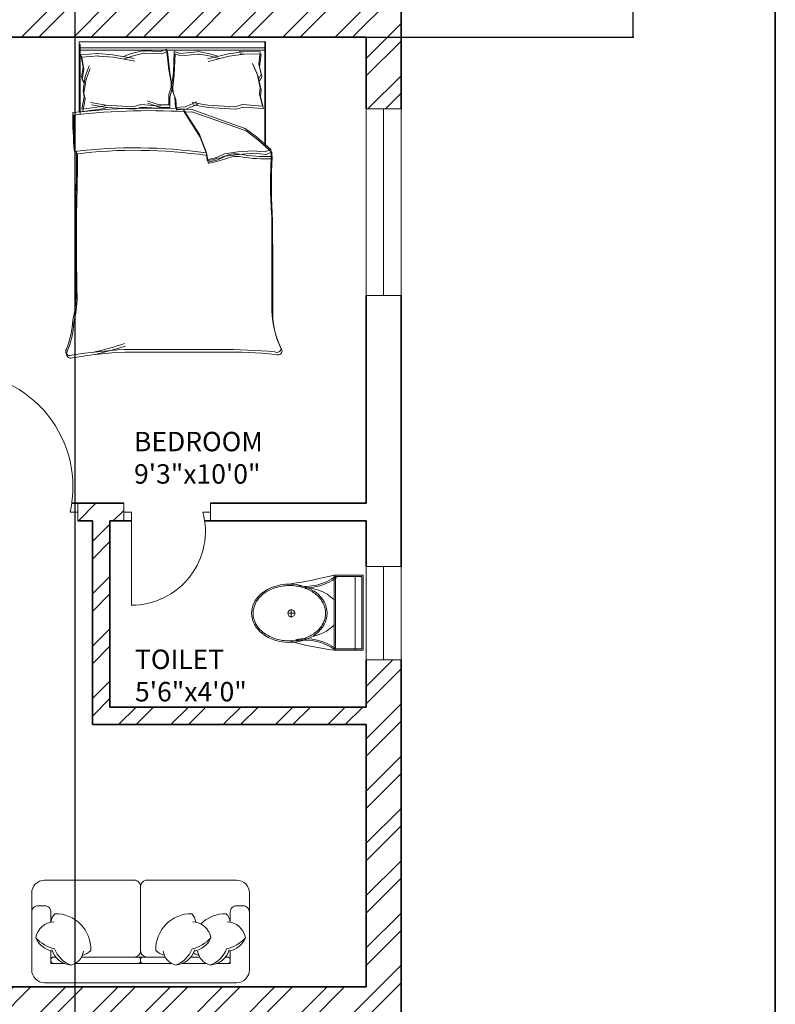
# Model space of a CAD drawing. Units: inches. Extents: x 2552 to 3217, y 1417 to 2737.
# Tile 13 of 25: x 3022 to 3217, y 1885 to 2138. Entities that reach past the tile are written whole.
import ezdxf

# ---------------------------------------------------------------- set-up
doc = ezdxf.new("R2010")
doc.units = ezdxf.units.IN
for name, color, linetype, lineweight in [('A-ANNO-DIMS', 2, 'Continuous', 18), ('A-ANNO-TTLB', 7, 'Continuous', 35), ('A-AREA-IDEN', 7, 'Continuous', 18), ('A-DOOR', 21, 'Continuous', 18), ('A-FLOR-FIXT', 8, 'Continuous', 18), ('A-FURN', 8, 'Continuous', 13), ('A-GLAZ', 161, 'Continuous', 18), ('A-WALL', 7, 'Continuous', 35), ('A-WALL-PATT', 217, 'Continuous', 13)]:
    doc.layers.add(name, color=color, linetype=linetype, lineweight=lineweight)
doc.styles.get("Standard").update_dxf_attribs({"font": 'arial.ttf'})
doc.dimstyles.get("Standard").update_dxf_attribs({"dimtxt": 0.18, "dimasz": 0.18, "dimexe": 0.18, "dimexo": 0.0625, "dimgap": 0.09, "dimtad": 0, "dimtih": 1, "dimtoh": 1, "dimdec": 4, "dimzin": 0, "dimdsep": 46, "dimtxsty": 'Standard', "dimcen": 0.09, "dimadec": 0, "dimazin": 0, "dimtfac": 1, "dimtdec": 4, "dimtofl": 0, "dimtmove": 0, "dimatfit": 3, "dimfxl": 1, "dimtolj": 1, "dimtzin": 0, "dimarcsym": 0})

# ---------------------------------------------------------------- blocks, each defined once
blk = doc.blocks.new('A$C31115884')
for p, q in [((283.1, 497.7), (223.4, 497.7)), ((257.5, 466.4), (257.5, 523.2)), ((0, 200), (0, 0)), ((520, 200), (0, 200)), ((10, 190), (10, 10)), ((510, 190), (10, 190)), ((510, 10), (510, 190)), ((520, 0), (520, 200)), ((510, 54.5), (0, 54.5)), ((10, 10), (510, 10)), ((0, 0), (520, 0))]:
    blk.add_line(p, q)
blk.add_circle((255.6, 496.4), 23.6)
for centre, radius, start, end in [((2777.7, -204.6), 2807, 165.4549, 171.71327), ((3237, 905), 2807, 188.28673, 194.5451), ((-294.5, 403.3), 364.7, 324.20913, 9.34987), ((-294.5, 403.3), 374.7, 324.20913, 9.34987), ((139.5, 406.2), 293.5, 315.84364, 2.65635), ((805.8, 403.3), 374.7, 179.20365, 215.79087), ((805.8, 403.3), 364.7, 170.65013, 215.79087), ((383.6, 406.2), 293.5, 190.27735, 224.15636)]:
    blk.add_arc(centre, radius, start, end)
blk.add_ellipse((256.2, 509.9), major_axis=(0, -260.7), ratio=0.772727)
blk.add_open_spline([(256.2, 259.2), (263.1, 259.2), (270, 259.7), (287.8, 262.3), (298.7, 265.1), (319.9, 273.1), (330.2, 278.4), (350.1, 291.1), (359.7, 298.7), (377.7, 315.9), (386.2, 325.5), (401.7, 346.6), (408.8, 358.1), (421.3, 382.5), (426.8, 395.5), (435.9, 422.4), (439.5, 436.4), (444.8, 465.1), (446.5, 479.7), (447.9, 509.2), (447.6, 524), (445, 553.3), (442.7, 567.8), (436.3, 596), (432.1, 609.7), (421.9, 636), (416, 648.6), (402.5, 672.1), (395, 683), (378.6, 703), (369.8, 712.1), (351.1, 728), (341.3, 734.8), (320.9, 746.2), (310.4, 750.7), (288.9, 757.3), (278, 759.4), (256, 761), (245, 760.6), (223.1, 757.2), (212.3, 754.3), (191.1, 746.1), (180.8, 740.7), (160.9, 727.8), (151.4, 720.1), (133.5, 702.7), (125.1, 693), (109.6, 671.7), (102.6, 660.2), (90.2, 635.7), (84.9, 622.7), (76, 595.6), (72.4, 581.6), (67.2, 552.9), (65.6, 538.2), (64.4, 508.8), (64.8, 494), (67.5, 464.7), (69.9, 450.2), (76.6, 422), (80.8, 408.3), (91.1, 382.2), (97.2, 369.7), (110.8, 346.3), (118.4, 335.4), (134.8, 315.6), (143.7, 306.7), (162.4, 290.9), (172.3, 284.2), (192.8, 273), (203.3, 268.6), (224.8, 262.2), (235.8, 260.2), (249.9, 259.3), (253, 259.2), (256.2, 259.2)], degree=3, knots=[0, 0, 0, 0, 0.110105, 0.110105, 0.285049, 0.285049, 0.459994, 0.459994, 0.634938, 0.634938, 0.809882, 0.809882, 0.984827, 0.984827, 1.159771, 1.159771, 1.334715, 1.334715, 1.50966, 1.50966, 1.684604, 1.684604, 1.859549, 1.859549, 2.034493, 2.034493, 2.209437, 2.209437, 2.384382, 2.384382, 2.559326, 2.559326, 2.73427, 2.73427, 2.909215, 2.909215, 3.084159, 3.084159, 3.259103, 3.259103, 3.434048, 3.434048, 3.608992, 3.608992, 3.783936, 3.783936, 3.958881, 3.958881, 4.133825, 4.133825, 4.30877, 4.30877, 4.483714, 4.483714, 4.658658, 4.658658, 4.833603, 4.833603, 5.008547, 5.008547, 5.183491, 5.183491, 5.358436, 5.358436, 5.53338, 5.53338, 5.708324, 5.708324, 5.883269, 5.883269, 6.058213, 6.058213, 6.233158, 6.233158, 6.283185, 6.283185, 6.283185, 6.283185])
blk = doc.blocks.new('BED-DOUBLE')
for p, q in [((3.47, 63.33), (3.47, 81.44)), ((3.47, 81.44), (51.49, 81.44)), ((3.48, 63.33), (3.48, 81.44)), ((51.27, 81.44), (51.27, 54.83)), ((51.27, 81.44), (51.27, 54.83)), ((51.49, 81.44), (51.49, 80.8)), ((3.47, 79.91), (51.27, 79.91)), ((3.48, 79.91), (51.27, 79.91)), ((3.7, 62.69), (3.7, 80.8)), ((3.7, 62.69), (3.7, 80.8)), ((3.7, 79.27), (51.49, 79.27)), ((3.7, 79.27), (51.49, 79.27)), ((16.88, 78.42), (19.77, 79.14)), ((16.88, 78.42), (19.77, 79.14)), ((19.77, 79.14), (20.09, 79.14)), ((19.77, 79.14), (20.09, 79.14)), ((20.09, 79.14), (24.54, 78.99)), ((20.09, 79.14), (24.54, 78.99)), ((24.54, 78.99), (25.98, 79.57)), ((24.54, 78.99), (25.98, 79.57)), ((24.77, 78.36), (26.21, 78.93)), ((24.77, 78.36), (26.21, 78.93)), ((25.98, 79.57), (26.56, 74.22)), ((25.98, 79.57), (26.56, 74.22)), ((26.21, 78.93), (26.79, 73.58)), ((26.21, 78.93), (26.79, 73.58)), ((27.98, 78.95), (27.73, 73.58)), ((27.98, 78.95), (27.73, 73.58)), ((29.46, 78.46), (27.98, 78.95)), ((29.46, 78.46), (27.98, 78.95)), ((33.88, 78.89), (29.46, 78.46)), ((33.88, 78.89), (29.46, 78.46)), ((34.2, 78.91), (33.88, 78.89)), ((34.2, 78.91), (33.88, 78.89)), ((37.14, 78.36), (34.2, 78.91)), ((37.14, 78.36), (34.2, 78.91)), ((45.71, 78.9), (41.91, 78.37)), ((45.71, 78.9), (41.91, 78.37)), ((50.11, 78.89), (44.71, 78.98)), ((44.71, 78.98), (45.71, 78.9)), ((50.11, 78.89), (44.71, 78.98)), ((44.71, 78.98), (45.71, 78.9)), ((50.11, 78.89), (49.73, 75.68)), ((50.11, 78.89), (49.73, 75.68)), ((51.49, 80.8), (51.49, 54.19)), ((51.49, 80.8), (51.49, 54.19)), ((3.89, 78.13), (4.47, 74.95)), ((3.89, 78.13), (4.47, 74.95)), ((3.9, 78.11), (8.18, 78.43)), ((3.9, 78.11), (8.18, 78.43)), ((4.12, 77.49), (4.7, 74.31)), ((4.12, 77.49), (4.7, 74.31)), ((4.13, 77.47), (8.41, 77.8)), ((4.13, 77.47), (8.41, 77.8)), ((8.18, 78.43), (8.28, 78.42)), ((8.18, 78.43), (8.28, 78.42)), ((8.28, 78.42), (12.11, 78.13)), ((8.28, 78.42), (12.11, 78.13)), ((8.41, 77.8), (8.51, 77.78)), ((8.41, 77.8), (8.51, 77.78)), ((8.51, 77.78), (12.34, 77.49)), ((8.51, 77.78), (12.34, 77.49)), ((12.11, 78.13), (17.6, 77.12)), ((12.11, 78.13), (17.6, 77.12)), ((12.34, 77.49), (17.83, 76.48)), ((12.34, 77.49), (17.83, 76.48)), ((14.85, 77.69), (16.88, 78.42)), ((14.85, 77.69), (16.88, 78.42)), ((15.08, 77.05), (17.11, 77.78)), ((15.08, 77.05), (17.11, 77.78)), ((17.11, 77.78), (20, 78.5)), ((17.11, 77.78), (20, 78.5)), ((20, 78.5), (20.32, 78.5)), ((20, 78.5), (20.32, 78.5)), ((20.32, 78.5), (24.77, 78.36)), ((20.32, 78.5), (24.77, 78.36)), ((28.21, 78.31), (27.96, 72.94)), ((28.21, 78.31), (27.96, 72.94)), ((29.68, 77.83), (28.21, 78.31)), ((29.68, 77.83), (28.21, 78.31)), ((34.11, 78.25), (29.68, 77.83)), ((34.11, 78.25), (29.68, 77.83)), ((34.43, 78.27), (34.11, 78.25)), ((34.43, 78.27), (34.11, 78.25)), ((37.36, 77.73), (34.43, 78.27)), ((37.36, 77.73), (34.43, 78.27)), ((41.91, 78.37), (36.49, 77.02)), ((41.91, 78.37), (36.5, 77.02)), ((42.14, 77.73), (36.72, 76.38)), ((42.14, 77.73), (36.72, 76.38)), ((39.2, 77.77), (37.14, 78.36)), ((39.2, 77.77), (37.14, 78.36)), ((39.43, 77.13), (37.36, 77.73)), ((39.43, 77.13), (37.36, 77.73)), ((45.94, 78.26), (42.14, 77.73)), ((45.94, 78.26), (42.14, 77.73)), ((50.34, 78.25), (44.94, 78.34)), ((44.94, 78.34), (45.94, 78.26)), ((50.34, 78.25), (44.94, 78.34)), ((44.94, 78.34), (45.94, 78.26)), ((50.34, 78.25), (49.96, 75.04)), ((50.34, 78.25), (49.96, 75.04)), ((4.47, 74.95), (4.04, 72.34)), ((4.47, 74.95), (4.04, 72.34)), ((4.7, 74.31), (4.27, 71.7)), ((4.7, 74.31), (4.27, 71.7)), ((5.05, 72.49), (6.06, 75.24)), ((5.05, 72.49), (6.06, 75.24)), ((5.28, 71.85), (6.29, 74.6)), ((5.28, 71.85), (6.29, 74.6)), ((26.56, 74.22), (27.14, 71.04)), ((26.56, 74.22), (27.14, 71.04)), ((26.79, 73.58), (27.37, 70.4)), ((26.79, 73.58), (27.37, 70.4)), ((27.73, 73.58), (27.35, 70.37)), ((27.73, 73.58), (27.35, 70.37)), ((49.31, 73.19), (48.13, 75.86)), ((49.31, 73.19), (48.13, 75.86)), ((49.54, 72.55), (48.36, 75.23)), ((49.54, 72.55), (48.36, 75.23)), ((49.73, 75.68), (50.33, 73.1)), ((49.73, 75.68), (50.33, 73.1)), ((49.96, 75.04), (50.56, 72.47)), ((49.96, 75.04), (50.56, 72.47)), ((4.04, 72.34), (4.62, 71.33)), ((4.04, 72.34), (4.62, 71.33)), ((4.27, 71.7), (4.85, 70.69)), ((4.27, 71.7), (4.85, 70.69)), ((4.47, 68.87), (5.05, 72.49)), ((4.47, 68.87), (5.05, 72.49)), ((4.7, 68.23), (5.28, 71.85)), ((4.7, 68.23), (5.28, 71.85)), ((27.14, 71.04), (27.14, 69.74)), ((27.14, 71.04), (27.14, 69.74)), ((27.96, 72.94), (27.58, 69.73)), ((27.96, 72.94), (27.58, 69.73)), ((50.11, 69.61), (49.31, 73.19)), ((50.11, 69.61), (49.31, 73.19)), ((50.34, 68.98), (49.54, 72.55)), ((50.34, 68.98), (49.54, 72.55)), ((50.33, 73.1), (49.81, 72.06)), ((50.33, 73.1), (49.81, 72.06)), ((50.56, 72.47), (50.04, 71.42)), ((50.56, 72.47), (50.04, 71.42)), ((4.76, 67.28), (4.47, 68.87)), ((4.76, 67.28), (4.47, 68.87)), ((27.14, 69.74), (26.56, 67.86)), ((27.14, 69.74), (26.56, 67.86)), ((27.37, 69.1), (26.79, 67.22)), ((27.37, 69.1), (26.79, 67.22)), ((27.35, 70.37), (27.44, 69.07)), ((27.35, 70.37), (27.44, 69.07)), ((27.37, 70.4), (27.37, 69.1)), ((27.37, 70.4), (27.37, 69.1)), ((27.44, 69.07), (28.13, 67.23)), ((27.44, 69.07), (28.13, 67.23)), ((27.58, 69.73), (27.66, 68.43)), ((27.58, 69.73), (27.66, 68.43)), ((49.92, 68.01), (50.11, 69.61)), ((49.92, 68.01), (50.11, 69.61)), ((50.15, 67.37), (50.34, 68.98)), ((50.15, 67.37), (50.34, 68.98)), ((4.18, 64.1), (4.76, 67.28)), ((4.18, 64.1), (4.76, 67.28)), ((4.41, 63.46), (4.99, 66.64)), ((4.41, 63.46), (4.99, 66.64)), ((4.99, 66.64), (4.7, 68.23)), ((4.99, 66.64), (4.7, 68.23)), ((24.1, 65.18), (20.96, 66.27)), ((24.1, 65.18), (20.96, 66.27)), ((26.56, 67.86), (26.56, 65.18)), ((26.56, 67.86), (26.56, 65.18)), ((26.79, 67.22), (26.79, 64.54)), ((26.79, 67.22), (26.79, 64.54)), ((27.66, 68.43), (28.36, 66.59)), ((27.66, 68.43), (28.36, 66.59)), ((28.13, 67.23), (28.3, 64.55)), ((28.13, 67.23), (28.3, 64.55)), ((28.36, 66.59), (28.53, 63.91)), ((28.36, 66.59), (28.53, 63.91)), ((30.75, 64.7), (33.82, 65.99)), ((30.75, 64.7), (33.82, 65.99)), ((50.7, 64.87), (49.92, 68.01)), ((50.7, 64.87), (49.92, 68.01)), ((50.93, 64.23), (50.15, 67.37)), ((50.93, 64.23), (50.15, 67.37)), ((9.28, 64.83), (4.18, 64.1)), ((9.28, 64.83), (4.18, 64.1)), ((9.51, 64.19), (4.41, 63.46)), ((9.51, 64.19), (4.41, 63.46)), ((6.38, 65.81), (10.41, 65.15)), ((6.38, 65.81), (10.41, 65.15)), ((6.61, 65.18), (10.64, 64.51)), ((6.61, 65.18), (10.64, 64.51)), ((10.41, 65.15), (9.28, 64.83)), ((10.41, 65.15), (9.28, 64.83)), ((10.64, 64.51), (9.51, 64.19)), ((10.64, 64.51), (9.51, 64.19)), ((10.41, 65.15), (17.42, 64.72)), ((10.41, 65.15), (17.42, 64.72)), ((10.64, 64.51), (17.65, 64.08)), ((10.64, 64.51), (17.65, 64.08)), ((17.42, 64.72), (19.38, 65.27)), ((17.42, 64.72), (19.38, 65.27)), ((17.65, 64.08), (19.61, 64.63)), ((17.65, 64.08), (19.61, 64.63)), ((19.38, 65.27), (24.52, 64.87)), ((19.38, 65.27), (24.52, 64.87)), ((19.61, 64.63), (24.74, 64.23)), ((19.61, 64.63), (24.74, 64.23)), ((24.33, 64.54), (21.19, 65.63)), ((24.33, 64.54), (21.19, 65.63)), ((26.56, 65.18), (24.1, 65.18)), ((26.56, 65.18), (24.1, 65.18)), ((26.79, 64.54), (24.33, 64.54)), ((26.79, 64.54), (24.33, 64.54)), ((28.3, 64.55), (30.75, 64.7)), ((28.3, 64.55), (30.75, 64.7)), ((28.53, 63.91), (30.98, 64.06)), ((28.53, 63.91), (30.98, 64.06)), ((30.26, 64.06), (34.45, 57.57)), ((30.26, 64.06), (34.45, 57.57)), ((30.49, 63.42), (34.68, 56.93)), ((30.49, 63.42), (34.68, 56.93)), ((30.98, 64.06), (34.05, 65.35)), ((30.98, 64.06), (34.05, 65.35)), ((40.64, 61.13), (32.31, 64.06)), ((40.64, 61.13), (32.31, 64.06)), ((40.87, 60.49), (32.53, 63.42)), ((40.87, 60.49), (32.53, 63.42)), ((32.56, 65.81), (36.6, 65.15)), ((32.56, 65.81), (36.6, 65.15)), ((32.79, 65.18), (36.82, 64.51)), ((32.79, 65.18), (36.82, 64.51)), ((36.6, 65.15), (43.61, 64.72)), ((36.6, 65.15), (43.61, 64.72)), ((36.82, 64.51), (43.83, 64.08)), ((36.82, 64.51), (43.83, 64.08)), ((43.61, 64.72), (45.57, 65.27)), ((43.61, 64.72), (45.57, 65.27)), ((43.83, 64.08), (45.79, 64.63)), ((43.83, 64.08), (45.79, 64.63)), ((45.57, 65.27), (50.7, 64.87)), ((45.57, 65.27), (50.7, 64.87)), ((45.79, 64.63), (50.93, 64.23)), ((45.79, 64.63), (50.93, 64.23)), ((46.22, 59.11), (40.64, 61.13)), ((46.22, 59.11), (40.64, 61.13)), ((46.45, 58.48), (40.87, 60.49)), ((46.45, 58.48), (40.87, 60.49)), ((49.16, 56.95), (46.22, 59.11)), ((49.16, 56.95), (46.22, 59.11)), ((49.39, 56.31), (46.45, 58.48)), ((49.39, 56.31), (46.45, 58.48)), ((34.45, 57.57), (36.15, 53.08)), ((34.45, 57.57), (36.15, 53.08)), ((34.68, 56.93), (36.38, 52.44)), ((34.68, 56.93), (36.38, 52.44)), ((52.87, 53.7), (49.16, 56.95)), ((52.87, 53.7), (49.16, 56.95)), ((53.1, 53.06), (49.39, 56.31)), ((53.1, 53.06), (49.39, 56.31)), ((44.36, 53.08), (48.23, 53.39)), ((44.36, 53.08), (48.23, 53.39)), ((48.23, 53.39), (51.33, 53.08)), ((48.23, 53.39), (51.33, 53.08)), ((51.33, 53.08), (52.87, 53.7)), ((51.33, 53.08), (52.87, 53.7)), ((52.95, 51.95), (52.87, 53.7, 3.87)), ((52.95, 51.95), (52.87, 53.7, 3.87)), ((36.15, 53.08), (36.46, 51.07)), ((36.15, 53.08), (36.46, 51.07)), ((36.38, 52.44), (36.69, 50.43)), ((36.38, 52.44), (36.69, 50.43)), ((36.46, 51.07), (38.94, 51.69)), ((36.46, 51.07), (38.94, 51.69)), ((36.69, 50.43), (39.17, 51.05)), ((36.69, 50.43), (39.17, 51.05)), ((38.94, 51.69), (40.95, 52.61)), ((38.94, 51.69), (40.95, 52.61)), ((39.17, 51.05), (41.18, 51.97)), ((39.17, 51.05), (41.18, 51.97)), ((40.95, 52.61), (44.36, 53.08)), ((40.95, 52.61), (44.36, 53.08)), ((41.18, 51.97), (44.59, 52.44)), ((41.18, 51.97), (44.59, 52.44)), ((44.59, 52.44), (48.46, 52.75)), ((44.59, 52.44), (48.46, 52.75)), ((48.46, 52.75), (51.56, 52.44)), ((48.46, 52.75), (51.56, 52.44)), ((51.56, 52.44), (53.1, 53.06)), ((51.56, 52.44), (53.1, 53.06)), ((53.18, 51.31), (53.1, 53.06, 3.87)), ((53.18, 51.31), (53.1, 53.06, 3.87)), ((15.06, 2.2), (39.68, 2.2)), ((15.06, 2.2), (39.68, 2.2)), ((15.29, 1.56), (39.91, 1.56)), ((15.29, 1.56), (39.91, 1.56))]:
    blk.add_line(p, q)
for centre, radius, start, end in [((21.36, -100.61), 164.97, 86.0865, 96.7821), ((21.36, -100.61), 164.97, 86.0865, 96.7821), ((21.59, -101.25), 164.97, 86.0865, 96.7821), ((21.59, -101.25), 164.97, 86.0865, 96.7821), ((85.16, 61.35), 83.31, 178.7218, 185.604), ((85.16, 61.35), 83.31, 178.7218, 185.604), ((85.39, 60.71), 83.31, 178.7218, 185.604), ((85.39, 60.71), 83.31, 178.7218, 185.604), ((17.76, -74.87), 129.02, 81.7845, 96.9006), ((17.76, -74.87), 129.02, 81.7845, 96.9006), ((17.98, -75.51), 129.02, 81.7845, 96.9006), ((17.98, -75.51), 129.02, 81.7845, 96.9006), ((-167.31, 50.27), 170.11, 358.4762, 1.0082), ((-167.31, 50.27), 170.11, 358.4762, 1.0082), ((-167.08, 49.63), 170.11, 358.4762, 1.0082), ((-167.08, 49.63), 170.11, 358.4762, 1.0082), ((36.64, 51), 0.185, 160.2464, 271.1377), ((36.64, 51), 0.185, 160.2464, 271.1377), ((31.15, 79.96), 29.65, 280.6617, 289.8806), ((31.15, 79.96), 29.65, 280.6617, 289.8806), ((31.38, 79.32), 29.65, 280.6617, 289.8806), ((31.38, 79.32), 29.65, 280.6617, 289.8806), ((43.74, 46.38), 6.22, 78.6608, 113.7384), ((43.74, 46.38), 6.22, 78.6608, 113.7384), ((43.97, 45.74), 6.22, 78.6608, 113.7384), ((43.97, 45.74), 6.22, 78.6608, 113.7384), ((51.33, 88.1), 36.18, 259.8763, 272.5657), ((51.33, 88.1), 36.18, 259.8763, 272.5657), ((51.56, 87.46), 36.18, 259.8763, 272.5657), ((51.56, 87.46), 36.18, 259.8763, 272.5657), ((182.27, 45.13), 129.5, 176.9791, 183.8365), ((182.27, 45.13), 129.5, 176.9791, 183.8365), ((182.49, 44.49), 129.5, 176.9791, 183.8365), ((182.49, 44.49), 129.5, 176.9791, 183.8365), ((36.86, 50.36), 0.185, 160.2464, 271.1377), ((36.86, 50.36), 0.185, 160.2464, 271.1377), ((484.82, 30.83), 482.31, 178.2277, 181.7185), ((484.82, 30.83), 482.31, 178.2277, 181.7185), ((485.05, 30.19), 482.31, 178.2277, 181.7185), ((485.05, 30.19), 482.31, 178.2277, 181.7185), ((-4508.74, 13.62), 4561.86, 0.00217, 0.28689), ((-4508.74, 13.62), 4561.86, 0.00217, 0.28689), ((-4508.51, 12.98), 4561.86, 0.00217, 0.28689), ((-4508.52, 12.98), 4561.86, 0.00217, 0.28689), ((-26.9, 16.93), 29.63, 346.0648, 358.9113), ((-26.9, 16.93), 29.63, 346.0648, 358.9113), ((-26.67, 16.29), 29.63, 346.0648, 358.9113), ((-26.67, 16.29), 29.63, 346.0648, 358.9113), ((76.16, 12.78), 23.07, 177.4714, 206.4681), ((76.16, 12.78), 23.07, 177.4714, 206.4681), ((76.39, 12.14), 23.07, 177.4714, 206.4681), ((76.39, 12.14), 23.07, 177.4714, 206.4681), ((-21.66, 11.17), 23.56, 337.9751, 356.652), ((-21.66, 11.17), 23.56, 337.9751, 356.652), ((-21.43, 10.53), 23.56, 337.9751, 356.652), ((-21.43, 10.53), 23.56, 337.9751, 356.652), ((-17.22, 105.16), 106.46, 283.3832, 287.7053), ((-17.22, 105.16), 106.46, 283.3832, 287.7053), ((-16.99, 104.52), 106.46, 283.3832, 287.7053), ((-16.99, 104.52), 106.46, 283.3832, 287.7053), ((1.09, 1.73), 1.09, 146.1736, 293.4781), ((1.09, 1.73), 1.09, 146.1736, 293.4781), ((1.32, 1.09), 1.09, 146.1736, 293.4781), ((1.32, 1.09), 1.09, 146.1736, 293.4781), ((21.43, -119.39), 121.76, 92.9958, 99.4091), ((21.43, -119.39), 121.76, 92.9958, 99.4091), ((21.66, -120.03), 121.76, 92.9958, 99.4091), ((21.65, -120.03), 121.76, 92.9958, 99.4091), ((41.15, -130.83), 133.04, 84.4998, 90.6351), ((41.15, -130.83), 133.04, 84.4998, 90.6351), ((41.38, -131.47), 133.04, 84.4998, 90.6351), ((41.38, -131.47), 133.04, 84.4998, 90.6351), ((54.41, 2.57), 1.1, 242.6588, 356.02), ((54.41, 2.57), 1.1, 242.6588, 356.02), ((54.64, 1.93), 1.1, 242.6588, 356.02), ((54.64, 1.93), 1.1, 242.6588, 356.02)]:
    blk.add_arc(centre, radius, start, end)
blk = doc.blocks.new('SOFA-WIDE')
at = {"ltscale": 0.03}
blk.add_lwpolyline([(26.39, 26.39, -0.414214), (28.04, 24.74, -0.414214), (29.69, 26.39), (52.79, 26.39, -0.414214), (56.08, 23.09), (56.08, 3.3, -0.414214), (52.79, 0), (3.3, 0, -0.414214), (0, 3.3), (0, 23.09, -0.414214), (3.3, 26.39), (26.39, 26.39, -0.414214), (28.04, 24.74, -0.414214), (29.69, 26.39)], format="xyb", dxfattribs=at)
for points in [[(26.39, 6.6, 0.414214), (28.04, 8.25), (28.04, 24.74, 0.414214)], [(29.69, 6.6, -0.414214), (28.04, 8.25), (28.04, 24.74, -0.414214)], [(0, 18.15, -0.414214), (1.65, 19.8), (3.3, 19.8, -0.414214), (4.95, 18.15), (4.95, 15.59)], [(4.94, 15.59, -0.165541), (5.97, 17.77, -0.425989), (15.23, 8.32, -0.121523), (13.03, 7.02, 7.115464)], [(42.25, 15.59, 0.165541), (41.23, 17.77, 0.425989), (31.97, 8.32, 0.121523), (34.17, 7.02, -7.115464)], [(51.14, 15.59, 0.165541), (50.12, 17.77, 0.200231), (43.57, 15.11, 0.121523)], [(51.14, 15.59), (51.14, 18.15, -0.414214), (52.79, 19.8), (54.44, 19.8, -0.414214), (56.08, 18.15)], [(5.78, 15.69, 0.356772), (1.05, 11.53, 0.249542), (5.33, 8.11, -9.61688)], [(41.42, 15.69, -0.356772), (46.15, 11.53, -0.249542), (41.87, 8.11, 9.61688)], [(50.31, 15.69, -0.356772), (55.04, 11.53, -0.249542), (50.75, 8.11, 9.61688)], [(1.05, 11.53, 0.14773), (5.87, 8.7, 0.213343), (10.12, 4.54, 0.178662)], [(46.15, 11.53, -0.14773), (41.33, 8.7, -0.213343), (37.07, 4.54, -0.178662)], [(55.04, 11.53, -0.14773), (50.21, 8.7, -0.213343), (45.96, 4.54, -0.178662)], [(5.2, 8.47, 0.306663), (10.12, 4.54, 0.30633), (13.34, 8.13, -0.872847)], [(26.39, 6.6, 0.414214), (28.04, 8.25)], [(29.69, 6.6, -0.414214), (28.04, 8.25)], [(41.99, 8.47, -0.306663), (37.07, 4.54, -0.30633), (33.86, 8.13, 0.872847)], [(41.67, 7.66, 0.071865), (43.05, 7.02, -7.115464)], [(50.88, 8.47, -0.306663), (45.96, 4.54, -0.30633), (42.75, 8.13, 0.872847)], [(47.67, 4.95), (51.14, 4.95), (51.14, 8.19, -0.414214)], [(6.21, 6.6), (5.61, 6.6, 0.414214), (4.95, 5.94), (4.95, 5.61, 0.414214), (5.61, 4.95)], [(11.16, 4.95), (27.38, 4.95, 0.414214), (28.04, 5.61), (28.04, 5.94, 0.414214), (27.38, 6.6), (12.82, 6.6, 0.414214)], [(36.04, 4.95), (28.7, 4.95, -0.414214), (28.04, 5.61), (28.04, 5.94, -0.414214), (28.7, 6.6), (34.37, 6.6, -0.414214)], [(40.99, 6.6), (43.26, 6.6, -0.414214)], [(49.88, 6.6), (50.48, 6.6, -0.414214), (51.14, 5.94), (51.14, 5.61, -0.414214), (50.48, 4.95)], [(5.61, 4.95), (8.42, 4.95, 0.414214)], [(44.92, 4.95), (38.78, 4.95, -0.414214)], [(50.48, 4.95), (47.67, 4.95, -0.414214)]]:
    blk.add_lwpolyline(points, format="xyb")
for points in [[(4.95, 8.19), (4.95, 4.95), (8.42, 4.95)], [(11.16, 4.95), (36.04, 4.95)], [(38.78, 4.95), (44.92, 4.95)]]:
    blk.add_lwpolyline(points)
blk.add_lwpolyline([(27.38, 4.95), (28.7, 4.95, -0.414214), (28.04, 5.61), (28.04, 5.94, -0.414214), (28.7, 6.6), (27.38, 6.6, -0.414214), (28.04, 5.94), (28.04, 5.61, -0.414214)], format="xyb", close=True)
blk = doc.blocks.new('WIN-48')
for p, q in [((4.5, 48), (0, 48)), ((0, 48), (9, 48)), ((0, 48), (0, 0)), ((4.5, 0), (4.5, 48)), ((9, 48), (9, 0)), ((0, 0), (9, 0)), ((9, 0), (4.5, 0))]:
    blk.add_line(p, q)
blk = doc.blocks.new('WIN-24')
for p, q in [((0, 24), (9, 24)), ((0, 24), (0, 0)), ((9, 24), (4.5, 24)), ((4.5, 24), (4.5, 0)), ((9, 24), (9, 0)), ((4.5, 0), (0, 0)), ((0, 0), (9, 0))]:
    blk.add_line(p, q)
blk = doc.blocks.new('*D54')
at = {"layer": 'A-ANNO-DIMS', "color": 0, "lineweight": -2, "transparency": 16777216}
for p, q in [((3111.42, 2387.01), (3180.33, 2387.01)), ((3180.15, 2386.83), (3180.15, 2260.44)), ((3180.15, 2133.69), (3180.15, 2260.08)), ((3111.42, 2133.51), (3180.33, 2133.51))]:
    blk.add_line(p, q, dxfattribs=at)
at = {"layer": 'A-ANNO-DIMS', "color": 0, "transparency": 16777216}
for points in [[(3180.12, 2386.83), (3180.18, 2386.83), (3180.15, 2387.01)], [(3180.12, 2133.69), (3180.18, 2133.69), (3180.15, 2133.51)]]:
    blk.add_solid(points, dxfattribs=at)
at = {"layer": 'Defpoints', "color": 0, "transparency": 16777216}
for p in [(3111.35, 2387.01), (3180.15, 2387.01), (3111.35, 2133.51)]:
    blk.add_point(p, dxfattribs=at)
at = {"layer": 'A-ANNO-DIMS', "color": 0, "transparency": 16777216, "insert": (3180.15, 2260.26), "char_height": 0.18, "attachment_point": 5}
blk.add_mtext('\\A1;253.5', dxfattribs=at)
blk = doc.blocks.new('*D57')
at = {"layer": 'A-ANNO-DIMS', "color": 0, "lineweight": -2, "transparency": 16777216}
for p, q in [((3004.08, 2515.95), (3004.08, 1482.53)), ((3036.34, 2515.95), (3036.34, 1482.53)), ((3004.26, 1482.71), (3019.75, 1482.71)), ((3036.16, 1482.71), (3020.68, 1482.71))]:
    blk.add_line(p, q, dxfattribs=at)
at = {"layer": 'A-ANNO-DIMS', "color": 0, "transparency": 16777216}
for points in [[(3004.26, 1482.74), (3004.26, 1482.68), (3004.08, 1482.71)], [(3036.16, 1482.74), (3036.16, 1482.68), (3036.34, 1482.71)]]:
    blk.add_solid(points, dxfattribs=at)
at = {"layer": 'Defpoints', "color": 0, "transparency": 16777216}
for p in [(3004.08, 2516.01), (3036.34, 2516.01), (3036.34, 1482.71)]:
    blk.add_point(p, dxfattribs=at)
at = {"layer": 'A-ANNO-DIMS', "color": 0, "transparency": 16777216, "insert": (3020.21, 1482.71), "char_height": 0.18, "attachment_point": 5}
blk.add_mtext('\\A1;32.255', dxfattribs=at)

msp = doc.modelspace()

# ---------------------------------------------------------------- hatches: boundary and pattern name
at = {"layer": 'A-WALL-PATT'}
h = msp.add_hatch(dxfattribs=at)
h.set_pattern_fill('ANSI32', color=256)
h.paths.add_polyline_path([(2756.676, 2649.5125), (2637.3535, 2649.5125), (2637.3535, 2617.9626), (2641.8535, 2617.9626), (2646.3535, 2617.9626), (2646.3535, 2640.5125), (2724.3535, 2640.5125), (2724.3535, 2520.5125), (2720.299, 2520.5125), (2720.299, 2516.0125), (2733.4075, 2516.0125), (2733.4075, 2518.2213), (2733.4075, 2520.5125), (2728.8535, 2520.5125), (2728.8535, 2640.5125), (2756.676, 2640.5125)])
h.paths.add_polyline_path([(2848.8535, 2649.5125), (2804.676, 2649.5125), (2804.676, 2640.5125), (2839.8535, 2640.5125), (2839.8535, 2598.3517), (2848.8535, 2598.3517)])
h.paths.add_polyline_path([(2646.3535, 2516.0125), (2697.9593, 2516.0125), (2697.9593, 2518.2625), (2697.9593, 2520.5125), (2646.3535, 2520.5125), (2646.3535, 2581.9626), (2637.3535, 2581.9626), (2637.3535, 2364.3298), (2646.3535, 2364.3298), (2646.3535, 2387.0125), (2724.3535, 2387.0125), (2724.3535, 2267.0125), (2721.0443, 2267.0125), (2721.0443, 2262.5125), (2733.7854, 2262.5125), (2733.7854, 2264.7625), (2733.7854, 2267.0125), (2728.8535, 2267.0125), (2728.8535, 2387.0125), (2839.8535, 2387.0125), (2839.8535, 2363.8387), (2848.8535, 2363.8387), (2848.8535, 2403.7415), (2844.3535, 2403.7415), (2839.8535, 2403.7415), (2839.8535, 2396.0125), (2646.3535, 2396.0125)])
h.paths.add_polyline_path([(2848.8535, 2550.3517), (2844.3535, 2550.3517), (2839.8535, 2550.3517), (2839.8535, 2520.5125), (2801.9195, 2520.5125), (2801.9195, 2518.2625), (2801.9195, 2516.0125), (2839.8535, 2516.0125), (2839.8535, 2507.5813), (2848.8535, 2507.5813)], flags=17)
h.paths.add_polyline_path([(2848.8535, 2483.5813), (2844.3535, 2483.5813), (2839.8535, 2483.5813), (2839.8535, 2468.0125), (2773.8535, 2468.0125), (2773.8535, 2516.0125), (2778.1336, 2516.0125), (2778.1336, 2520.5125), (2766.696, 2520.5125), (2766.696, 2518.2625), (2766.696, 2516.0125), (2769.3535, 2516.0125), (2769.3535, 2463.5125), (2839.8535, 2463.5125), (2839.8535, 2431.0782), (2848.8535, 2431.0782)], flags=17)
h.paths.add_polyline_path([(2917.8535, 2569.2764), (2913.3535, 2569.2764), (2908.8535, 2569.2764), (2908.8535, 2433.001), (2917.8535, 2433.001), (2917.8535, 2516.0125), (2967.486, 2516.0125), (2967.486, 2520.5125), (2917.8535, 2520.5125)])
h.paths.add_polyline_path([(3000.3535, 2640.5125), (2995.8535, 2640.5125), (2995.8535, 2520.5125), (2990.688, 2520.5125), (2990.688, 2516.0125), (3004.0844, 2516.0125), (3004.0844, 2518.2625), (3004.0844, 2520.5125), (3000.3535, 2520.5125)])
h.paths.add_polyline_path([(3120.3535, 2561.3689), (3115.8535, 2561.3689), (3111.3535, 2561.3689), (3111.3535, 2520.5125), (3070.9814, 2520.5125), (3070.9814, 2518.2625), (3070.9814, 2516.0125), (3111.3535, 2516.0125), (3111.3535, 2505.1841), (3120.3535, 2505.1841)])
h.paths.add_polyline_path([(3120.3535, 2481.1841), (3115.8535, 2481.1841), (3111.3535, 2481.1841), (3111.3535, 2468.0125), (3045.3535, 2468.0125), (3045.3535, 2516.0125), (3048.9787, 2516.0125), (3048.9787, 2520.5125), (3036.3395, 2520.5125), (3036.3395, 2516.0125), (3040.8535, 2516.0125), (3040.8535, 2463.5125), (3111.3535, 2463.5125), (3111.3535, 2396.0125), (2917.8535, 2396.0125), (2917.8535, 2403.4124), (2913.3535, 2403.4124), (2908.8535, 2403.4124), (2908.8535, 2182.5756), (2917.8535, 2182.5756), (2917.8535, 2262.5125), (2968.001, 2262.5125), (2968.001, 2264.7625), (2968.001, 2267.0125), (2917.8535, 2267.0125), (2917.8535, 2387.0125), (3111.3535, 2387.0125), (3111.3535, 2352.2435), (3120.3535, 2352.2435)])
h.paths.add_polyline_path([(3120.3535, 2304.2435), (3115.8535, 2304.2435), (3111.3535, 2304.2435), (3111.3535, 2267.0125), (3073.8616, 2267.0125), (3073.8616, 2264.7625), (3073.8616, 2262.5125), (3111.3535, 2262.5125), (3111.3535, 2252.376), (3120.3535, 2252.376)], flags=17)
h.paths.add_polyline_path([(3120.3535, 2228.376), (3115.8535, 2228.376), (3111.3535, 2228.376), (3111.3535, 2214.5125), (3045.3535, 2214.5125), (3045.3535, 2262.5125), (3049.3096, 2262.5125), (3049.3096, 2267.0125), (3035.0125, 2267.0125), (3035.0125, 2262.5125), (3040.8535, 2262.5125), (3040.8535, 2210.0125), (3111.3535, 2210.0125), (3111.3535, 2142.5125), (2917.8535, 2142.5125), (2917.8535, 2150.2408), (2913.3535, 2150.2408), (2908.8535, 2150.2408), (2908.8535, 1924.9905), (2917.8535, 1924.9905), (2917.8535, 2009.0125), (2971.959, 2009.0125), (2971.959, 2011.2625), (2971.959, 2013.5125), (2917.8535, 2013.5125), (2917.8535, 2133.5125), (2995.8535, 2133.5125), (2995.8535, 2013.5125), (2992.1797, 2013.5125), (2992.1797, 2009.0125), (3004.3344, 2009.0125), (3004.3344, 2011.2625), (3004.3344, 2013.5125), (3000.3535, 2013.5125), (3000.3535, 2133.5125), (3111.3535, 2133.5125), (3111.3535, 2115.0291), (3120.3535, 2115.0291)])
h.paths.add_polyline_path([(3000.3535, 2387.0125), (2995.8535, 2387.0125), (2995.8535, 2267.0125), (2991.3326, 2267.0125), (2991.3326, 2262.5125), (3004.1044, 2262.5125), (3004.1044, 2264.7625), (3004.1044, 2267.0125), (3000.3535, 2267.0125)], flags=17)
h.paths.add_polyline_path([(3120.3535, 1973.2388), (3115.8535, 1973.2388), (3111.3535, 1973.2388), (3111.3535, 1961.0125), (3045.3535, 1961.0125), (3045.3535, 2009.0125), (3048.9101, 2009.0125), (3048.9101, 2013.5125), (3037.105, 2013.5125), (3037.105, 2011.2625), (3037.105, 2009.0125), (3040.8535, 2009.0125), (3040.8535, 1956.5125), (3111.3535, 1956.5125), (3111.3535, 1889.0125), (2917.8535, 1889.0125), (2917.8535, 1895.7215), (2913.3535, 1895.7215), (2908.8535, 1895.7215), (2908.8535, 1844.2217), (2917.8535, 1844.2217), (2917.8535, 1880.0125), (3111.3535, 1880.0125), (3111.3535, 1846.9541), (3120.3535, 1846.9541)])
h.paths.add_polyline_path([(3120.3535, 2067.0291), (3111.3535, 2067.0291), (3111.3535, 2013.5125), (3071.3001, 2013.5125), (3071.3001, 2009.0125), (3111.3535, 2009.0125), (3111.3535, 1997.2388), (3120.3535, 1997.2388)], flags=0)
h.paths.add_polyline_path([(3120.3535, 1798.9541), (3115.8535, 1798.9541), (3111.3535, 1798.9541), (3111.3535, 1760.0125), (3071.2497, 1760.0125), (3071.2497, 1757.7625), (3071.2497, 1755.5125), (3111.3535, 1755.5125), (3111.3535, 1746.162), (3120.3535, 1746.2478)])
h.paths.add_polyline_path([(3120.3535, 1722.2049), (3111.3535, 1722.2049), (3111.3535, 1707.5125), (3045.3535, 1707.5125), (3045.3535, 1755.5125), (3048.6624, 1755.5125), (3048.6624, 1760.0125), (3035.3703, 1760.0125), (3035.3703, 1755.5125), (3040.8535, 1755.5125), (3040.8535, 1703.0125), (3111.3535, 1703.0125), (3111.3535, 1635.5125), (2917.8535, 1635.5125), (2917.8535, 1643.1366), (2913.3535, 1643.1366), (2908.8535, 1643.1366), (2908.8535, 1626.5125), (3120.3535, 1626.5125)])
h.paths.add_polyline_path([(2917.8535, 1755.5125), (2973.2287, 1755.5125), (2973.2287, 1757.7625), (2973.2287, 1760.0125), (2917.8535, 1760.0125), (2917.8535, 1808.2217), (2913.3535, 1808.2217), (2908.8535, 1808.2217), (2908.8535, 1676.1665), (2917.8535, 1676.1665)])
h.paths.add_polyline_path([(3000.3535, 1880.0125), (2995.8535, 1880.0125), (2995.8535, 1760.0125), (2992.9329, 1760.0125), (2992.9329, 1755.5125), (3003.8766, 1755.5125), (3003.8766, 1757.7625), (3003.8766, 1760.0125), (3000.3535, 1760.0125)])
h.paths.add_polyline_path([(2848.8535, 1896.6971), (2844.3535, 1896.6971), (2839.8535, 1896.6971), (2839.8535, 1889.0125), (2646.3535, 1889.0125), (2646.3535, 2009.0125), (2700.5253, 2009.0125), (2700.5253, 2011.2625), (2700.5253, 2013.5125), (2646.3535, 2013.5125), (2646.3535, 2053.1812), (2641.8535, 2053.1812), (2637.3535, 2053.1812), (2637.3535, 1836.254), (2646.3535, 1836.254), (2646.3535, 1880.0125), (2724.3535, 1880.0125), (2724.3535, 1760.0125), (2721.2473, 1760.0125), (2721.2473, 1755.5125), (2731.9187, 1755.5125), (2731.9187, 1757.7625), (2731.9187, 1760.0125), (2728.8535, 1760.0125), (2728.8535, 1880.0125), (2839.8535, 1880.0125), (2839.8535, 1840.3813), (2848.8535, 1840.3813)])
h.paths.add_polyline_path([(2848.8535, 1792.3813), (2844.3535, 1792.3813), (2839.8535, 1792.3813), (2839.8535, 1760.0125), (2797.8845, 1760.0125), (2797.8845, 1755.5125), (2839.8535, 1755.5125), (2839.8535, 1743.3688), (2844.3535, 1743.3688), (2848.8535, 1743.3688)], flags=0)
h.paths.add_polyline_path([(2848.8535, 1719.3688), (2844.3535, 1719.3688), (2839.8535, 1719.3688), (2839.8535, 1707.5125), (2773.8535, 1707.5125), (2773.8535, 1755.5125), (2777.716, 1755.5125), (2777.716, 1760.0125), (2760.9247, 1760.0125), (2760.9247, 1757.9721), (2760.9247, 1755.5125), (2769.3535, 1755.5125), (2769.3535, 1703.0125), (2839.8535, 1703.0125), (2839.8535, 1673.0277), (2848.8535, 1672.9407)], flags=0)
h.paths.add_polyline_path([(2646.3535, 1755.5125), (2702.9171, 1755.5125), (2702.9171, 1757.7625), (2702.9171, 1760.0125), (2646.3535, 1760.0125), (2646.3535, 1800.254), (2641.8535, 1800.254), (2637.3535, 1800.254), (2637.3535, 1626.5125), (2848.8535, 1626.5125), (2848.8535, 1643.1187), (2844.3535, 1643.1187), (2839.8535, 1643.1187), (2839.8535, 1635.5125), (2646.3535, 1635.5125)])
h.paths.add_polyline_path([(2848.8535, 2148.8427), (2844.3535, 2148.8427), (2839.8535, 2148.8427), (2839.8535, 2142.5125), (2646.3535, 2142.5125), (2646.3535, 2262.5125), (2701.3562, 2262.5125), (2701.3562, 2264.7625), (2701.3562, 2267.0125), (2646.3535, 2267.0125), (2646.3535, 2328.3298), (2637.3535, 2328.3298), (2637.3535, 2089.1812), (2646.3535, 2089.1812), (2646.3535, 2133.5125), (2839.8535, 2133.5125), (2839.8535, 2097.5966), (2848.8535, 2097.5966)])
h.paths.add_polyline_path([(2728.8535, 2133.5125), (2724.3535, 2133.5125), (2724.3535, 2013.5125), (2719.6039, 2013.5125), (2719.6039, 2009.0125), (2732.5784, 2009.0125), (2732.5784, 2011.2625), (2732.5784, 2013.5125), (2728.8535, 2013.5125)])
h.paths.add_polyline_path([(2848.8535, 1970.0557), (2844.3535, 1970.0557), (2839.8535, 1970.0557), (2839.8535, 1961.0125), (2773.8535, 1961.0125), (2773.8535, 2009.0125), (2777.3388, 2009.0125), (2777.3388, 2013.5125), (2764.7681, 2013.5125), (2764.7681, 2009.0125), (2769.3535, 2009.0125), (2769.3535, 1956.5125), (2839.8535, 1956.5125), (2839.8535, 1924.7199), (2848.8535, 1924.7199)], flags=17)
h.paths.add_polyline_path([(2848.8535, 2049.5966), (2844.3535, 2049.5966), (2839.8535, 2049.5966), (2839.8535, 2013.5125), (2798.198, 2013.5125), (2798.198, 2011.2625), (2798.198, 2009.0125), (2839.8535, 2009.0125), (2839.8535, 1994.0557), (2848.8535, 1994.0557)], flags=17)
h.paths.add_polyline_path([(2848.8535, 2315.8387), (2839.8535, 2315.8387), (2839.8535, 2267.0125), (2799.3375, 2267.0125), (2799.3375, 2264.7625), (2799.3375, 2262.5125), (2839.8535, 2262.5125), (2839.8535, 2253.2843), (2848.8535, 2253.2843)], flags=17)
h.paths.add_polyline_path([(2848.8535, 2229.2843), (2839.8535, 2229.2843), (2839.8535, 2177.6936), (2848.8535, 2177.6936)], flags=17)
h.paths.add_polyline_path([(2839.8535, 2214.5125), (2773.8535, 2214.5125), (2773.8535, 2262.5125), (2777.6984, 2262.5125), (2777.6984, 2267.0125), (2763.8226, 2267.0125), (2763.8226, 2262.5125), (2769.3535, 2262.5125), (2769.3535, 2210.0125), (2839.8535, 2210.0125)], flags=17)
h.paths.add_polyline_path([(3050.32, 2520.2817), (3088.9114, 2520.2817), (3088.9114, 2538.939), (3050.32, 2538.939)], flags=9)

# ---------------------------------------------------------------- linework, layer by layer
at = {"layer": 'A-ANNO-TTLB'}
msp.add_lwpolyline([(2552.473, 2736.5692), (3216.7862, 2736.5692), (3216.7862, 1416.6914), (2552.473, 1416.6914)], close=True, dxfattribs=at)
at = {"layer": 'A-DOOR'}
for p, q in [((3037.105, 2009.0125), (3037.105, 2013.5125)), ((3037.105, 2013.5125), (3037.105, 2011.2625)), ((3048.9101, 2009.0125), (3048.9101, 2013.5125)), ((3048.9101, 2013.5125), (3048.9101, 2011.2625)), ((3071.3001, 2013.5125), (3071.3001, 2009.0125)), ((3037.105, 2011.2625), (3035.105, 2011.2625)), ((3048.9101, 2011.2625), (3050.9101, 2011.2625)), ((3050.9101, 2011.2625), (3050.9101, 1987.2625)), ((3071.3001, 2011.2625), (3069.3001, 2011.2625)), ((3071.3001, 2009.0125), (3071.3001, 2011.2625))]:
    msp.add_line(p, q, dxfattribs=at)
for centre, radius, start, end in [((3006.3344, 2017.766), 29.4965, 347.262555, 90), ((3050.9101, 2006.3082), 19.0457, 270, 15.077614)]:
    msp.add_arc(centre, radius, start, end, dxfattribs=at)
at = {"layer": 'A-GLAZ'}
msp.add_line((3111.3535, 2115.0291), (3111.3535, 2115.0291), dxfattribs=at)
at = {"layer": 'A-WALL'}
for p, q in [((3120.3535, 2228.376), (3120.3535, 2115.0291)), ((3000.3535, 2133.5125), (3111.3535, 2133.5125)), ((3111.3535, 2133.5125), (3111.3535, 2115.0291)), ((3111.3535, 2067.0291), (3111.3535, 2013.5125)), ((3120.3535, 2067.0291), (3120.3535, 1997.2388)), ((3035.5226, 2013.5125), (3048.9101, 2013.5125)), ((3071.3001, 2013.5125), (3111.3535, 2013.5125)), ((3037.105, 2009.0125), (3040.8535, 2009.0125)), ((3040.8535, 2009.0125), (3040.8535, 1956.5125)), ((3045.3535, 2009.0125), (3045.3535, 1961.0125)), ((3045.3535, 2009.0125), (3050.9101, 2009.0125)), ((3069.7628, 2009.0125), (3111.3535, 2009.0125)), ((3111.3535, 2009.0125), (3111.3535, 1997.2388)), ((3111.3535, 1973.2388), (3111.3535, 1961.0125)), ((3120.3535, 1973.2388), (3120.3535, 1846.9541)), ((3045.3535, 1961.0125), (3111.3535, 1961.0125)), ((3040.8535, 1956.5125), (3111.3535, 1956.5125)), ((3111.3535, 1956.5125), (3111.3535, 1889.0125)), ((2917.8535, 1889.0125), (3111.3535, 1889.0125))]:
    msp.add_line(p, q, dxfattribs=at)

# ---------------------------------------------------------------- block references
at = {"layer": 'A-FLOR-FIXT', "xscale": 0.0372717239612423, "yscale": 0.0372717239612423, "zscale": 0.0372717239612423, "rotation": 89.99999999999999}
msp.add_blockref('A$C31115884', (3110.5924, 1975.6564), dxfattribs=at)
at = {"layer": 'A-FURN'}
for name, p in [('BED-DOUBLE', (3033.9717, 2050.8756)), ('SOFA-WIDE', (3025.2162, 1890.0773))]:
    msp.add_blockref(name, p, dxfattribs=at)
at = {"layer": 'A-GLAZ', "extrusion": (0, 0, -1), "zscale": -1, "rotation": 180}
for name, p in [('WIN-48', (-3111.354, 2115.0287)), ('WIN-24', (-3111.354, 1997.2391))]:
    msp.add_blockref(name, p, dxfattribs=at)

# ---------------------------------------------------------------- texts
at = {"layer": 'A-AREA-IDEN', "char_height": 5, "attachment_point": 1}
for s, width, insert in [('BEDROOM\\P9\'3"x10\'0"', 86.578964, (3051.5695, 2031.9011)), ('TOILET\\P5\'6"x4\'0"', 91.170993, (3051.8238, 1975.8363))]:
    msp.add_mtext_dynamic_manual_height_columns(s, width=width, gutter_width=12.5, heights=[0], dxfattribs=dict(at, insert=insert))

# ---------------------------------------------------------------- dimensions: what is measured, and where the dimension line sits
at = {"layer": 'A-ANNO-DIMS'}
dim = msp.add_linear_dim(base=(3036.3395, 1482.7125), p1=(3004.0844, 2516.0125), p2=(3036.3395, 2516.0125), dimstyle='Standard', override={"dimdec": 3, "dimlfac": 1, "dimrnd": 0, "dimzin": 0, "dimdsep": 46, "dimlunit": 2}, dxfattribs=at)
dim.commit()
dim.dimension.update_dxf_attribs({"geometry": '*D57', "text_midpoint": (3020.212, 1482.7125)})
dim = msp.add_linear_dim(base=(3180.1535, 2387.0125), p1=(3111.3535, 2133.5125), p2=(3111.3535, 2387.0125), angle=90, dimstyle='Standard', override={"dimdec": 1, "dimlfac": 1, "dimrnd": 0, "dimzin": 0, "dimdsep": 46, "dimlunit": 2}, dxfattribs=at)
dim.commit()
dim.dimension.update_dxf_attribs({"geometry": '*D54', "text_midpoint": (3180.1535, 2260.2625)})

doc.saveas('drawing.dxf')
